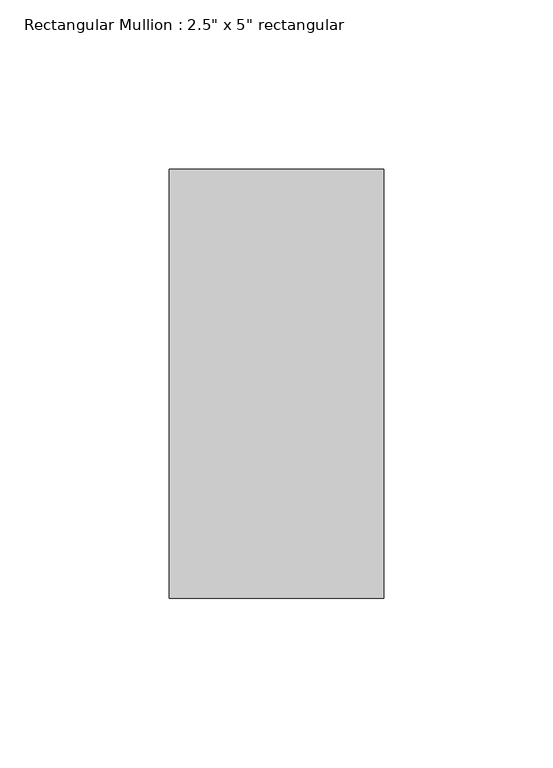
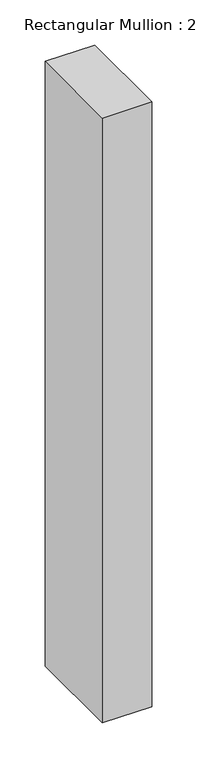
"""IFC4 building model written with IfcOpenShell, lengths in millimetres: member geometry."""

from ifc_helpers import new_model, si_unit, frame, origin, place, context, project, spatial, polyline, outline, extrude, source, transform, mapped, element, save


def member_c17f1be2(model_context):
    return source(origin(), model_context, "Body", "SweptSolid", [
        extrude(outline(polyline([(0.0, 63.5), (0.0, -63.5), (-63.5, -63.5), (-63.5, 63.5), (0.0, 63.5)])), frame((0.0, 0.0, -819.15), z_axis=(0.0, 0.0, 1.0), x_axis=(1.0, 0.0, 0.0)), (0.0, 0.0, 1.0), 819.15),
    ])


if __name__ == "__main__":
    model = new_model("IFC4")
    model_context = context("Model", 3, world=origin())
    ifc_project = project(units=[si_unit("LENGTHUNIT", "METRE", prefix="MILLI")], contexts=[model_context])
    site = spatial("IfcSite", under=ifc_project)
    building = spatial("IfcBuilding", under=site)
    placement = place(None, origin())
    member_shape = member_c17f1be2(model_context)
    element("IfcMember", 1, ObjectType="Rectangular Mullion : 2.5\" x 5\" rectangular", at=placement, inside=building, context=model_context, shape_type="MappedRepresentation", body=[
        mapped(member_shape, transform((0.0, 0.0, 0.0), x_axis=(1.0, 0.0, 0.0), y_axis=(0.0, 1.0, 0.0), z_axis=(0.0, 0.0, 1.0))),
    ])
    save(model, "model.ifc")

# Revit data of these elements
# Type "Rectangular Mullion : 2.5\" x 5\" rectangular"
#   built-in parameter 1007304 = 0.416667 (stored number, unit not read)
#   built-in parameter 1007301 = 0.104167 (stored number, unit not read)
#   built-in parameter 1007300 = 0.104167 (stored number, unit not read)
# Element 1 (IfcMember, "Rectangular Mullion : 2.5\" x 5\" rectangular")
#   Materials on its faces: "Iron, Ductile"
# Materials
#   "Iron, Ductile": class "Metal", colour RGB 0 0 0, transparency 0, Description = "Ductile cast iron", Cost = 0
